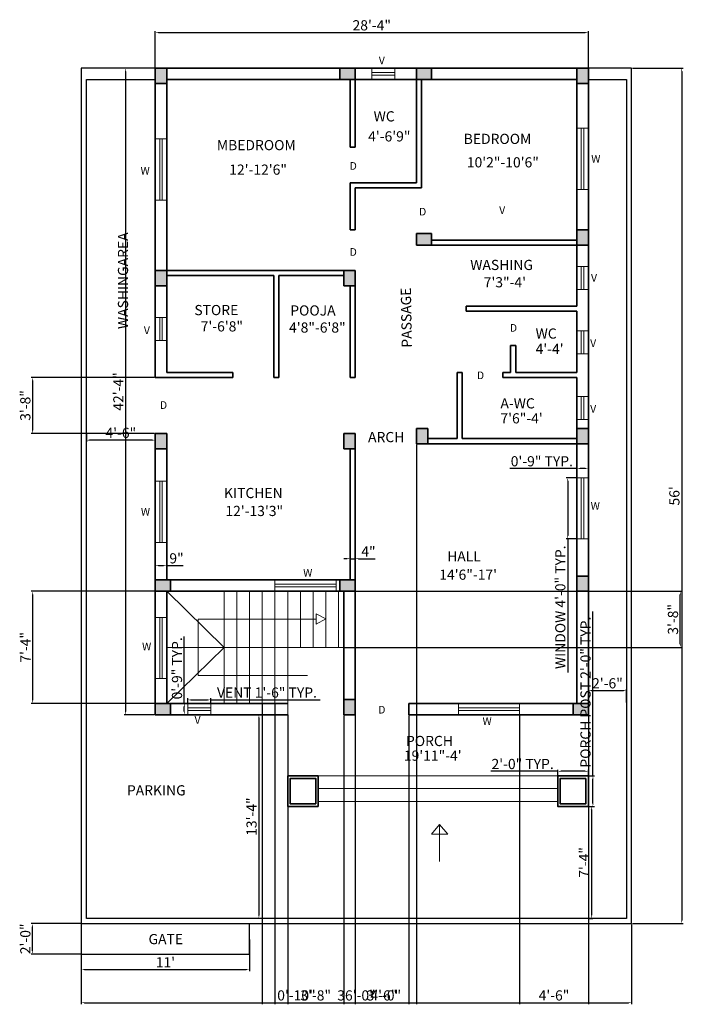
# Model space of a CAD drawing. Units: inches. Extents: x 2503 to 3024, y 1488 to 2262.
import ezdxf

# ---------------------------------------------------------------- set-up
doc = ezdxf.new("R2010")
doc.units = ezdxf.units.IN
for name, color, linetype, lineweight in [('A-ANNO-DIMS', 7, 'Continuous', 18), ('A-ANNO-SYMB', 121, 'Continuous', 18), ('A-ANNO-TEXT', 2, 'Continuous', 18), ('A-AREA-IDEN', 2, 'Continuous', 18), ('A-COLS', 121, 'Continuous', 35), ('A-COLS-PATT', 240, 'Continuous', 13), ('A-FLOR', 121, 'Continuous', 25), ('A-FLOR-STRS', 121, 'Continuous', 18), ('A-GLAZ', 6, 'Continuous', 18), ('A-WALL', 121, 'Continuous', 35), ('C-PROP', 121, 'Continuous', 25), ('C-SITE-GATE', 121, 'Continuous', 25)]:
    doc.layers.add(name, color=color, linetype=linetype, lineweight=lineweight)
doc.styles.get("Standard").update_dxf_attribs({"font": 'arial.ttf'})
doc.dimstyles.new('ISO-25', dxfattribs={"dimtxt": 8, "dimasz": 2.5, "dimexe": 1.25, "dimexo": 0.625, "dimtad": 1, "dimdec": 0, "dimlunit": 3, "dimtxsty": 'Standard', "dimcen": 2.5, "dimadec": 0, "dimazin": 0, "dimtfac": 1, "dimtdec": 0, "dimtmove": 0, "dimatfit": 3, "dimfxl": 1, "dimarcsym": 0})

# ---------------------------------------------------------------- blocks, each defined once
blk = doc.blocks.new('*D1')
at = {"layer": 'A-ANNO-DIMS', "color": 0, "lineweight": -2, "transparency": 16777216}
for p, q in [((2609.44, 2224.16), (2609.44, 2252.71)), ((2611.94, 2251.46), (2946.94, 2251.46)), ((2949.44, 2224.16), (2949.44, 2252.71))]:
    blk.add_line(p, q, dxfattribs=at)
at = {"layer": 'A-ANNO-DIMS', "color": 0, "transparency": 16777216}
for points in [[(2611.94, 2251.87), (2611.94, 2251.04), (2609.44, 2251.46)], [(2946.94, 2251.87), (2946.94, 2251.04), (2949.44, 2251.46)]]:
    blk.add_solid(points, dxfattribs=at)
at = {"layer": 'Defpoints', "color": 0, "transparency": 16777216}
for p in [(2949.44, 2251.46), (2609.44, 2223.53), (2949.44, 2223.53)]:
    blk.add_point(p, dxfattribs=at)
at = {"layer": 'A-ANNO-DIMS', "color": 0, "transparency": 16777216, "insert": (2779.44, 2256.17), "char_height": 8, "attachment_point": 5}
blk.add_mtext('28\'-4"', dxfattribs=at)
blk = doc.blocks.new('*D2')
at = {"layer": 'A-ANNO-DIMS', "color": 0, "lineweight": -2, "transparency": 16777216}
for p, q in [((2608.81, 2223.53), (2584.96, 2223.53)), ((2586.21, 2221.03), (2586.21, 1718.03)), ((2608.81, 1715.53), (2584.96, 1715.53))]:
    blk.add_line(p, q, dxfattribs=at)
at = {"layer": 'A-ANNO-DIMS', "color": 0, "transparency": 16777216}
for points in [[(2585.79, 2221.03), (2586.63, 2221.03), (2586.21, 2223.53)], [(2585.79, 1718.03), (2586.63, 1718.03), (2586.21, 1715.53)]]:
    blk.add_solid(points, dxfattribs=at)
at = {"layer": 'Defpoints', "color": 0, "transparency": 16777216}
for p in [(2609.44, 2223.53), (2586.21, 1715.53), (2609.44, 1715.53)]:
    blk.add_point(p, dxfattribs=at)
at = {"layer": 'A-ANNO-DIMS', "color": 0, "transparency": 16777216, "insert": (2581.57, 1969.53), "char_height": 8, "attachment_point": 5, "rotation": 90}
blk.add_mtext('42\'-4"', dxfattribs=at)
blk = doc.blocks.new('*D3')
at = {"layer": 'A-ANNO-DIMS', "color": 0, "lineweight": -2, "transparency": 16777216}
for p, q in [((2555.44, 1935.91), (2555.44, 1930.03)), ((2609.44, 1935.91), (2609.44, 1930.03)), ((2606.94, 1931.28), (2557.94, 1931.28))]:
    blk.add_line(p, q, dxfattribs=at)
at = {"layer": 'A-ANNO-DIMS', "color": 0, "transparency": 16777216}
for points in [[(2557.94, 1931.7), (2557.94, 1930.87), (2555.44, 1931.28)], [(2606.94, 1931.7), (2606.94, 1930.87), (2609.44, 1931.28)]]:
    blk.add_solid(points, dxfattribs=at)
at = {"layer": 'Defpoints', "color": 0, "transparency": 16777216}
for p in [(2555.44, 1936.53), (2609.44, 1936.53), (2555.44, 1931.28)]:
    blk.add_point(p, dxfattribs=at)
at = {"layer": 'A-ANNO-DIMS', "color": 0, "transparency": 16777216, "insert": (2582.44, 1935.99), "char_height": 8, "attachment_point": 5}
blk.add_mtext('4\'-6"', dxfattribs=at)
blk = doc.blocks.new('*D4')
at = {"layer": 'A-ANNO-DIMS', "color": 0, "lineweight": -2, "transparency": 16777216}
for p, q in [((2700.37, 1715.53), (2689.58, 1715.53)), ((2690.83, 1713.03), (2690.83, 1558.03)), ((2700.37, 1555.53), (2689.58, 1555.53))]:
    blk.add_line(p, q, dxfattribs=at)
at = {"layer": 'A-ANNO-DIMS', "color": 0, "transparency": 16777216}
for points in [[(2690.41, 1713.03), (2691.24, 1713.03), (2690.83, 1715.53)], [(2690.41, 1558.03), (2691.24, 1558.03), (2690.83, 1555.53)]]:
    blk.add_solid(points, dxfattribs=at)
at = {"layer": 'Defpoints', "color": 0, "transparency": 16777216}
for p in [(2700.99, 1715.53), (2690.83, 1555.53), (2700.99, 1555.53)]:
    blk.add_point(p, dxfattribs=at)
at = {"layer": 'A-ANNO-DIMS', "color": 0, "transparency": 16777216, "insert": (2686.11, 1635.53), "char_height": 8, "attachment_point": 5, "rotation": 90}
blk.add_mtext('13\'-4"', dxfattribs=at)
blk = doc.blocks.new('*D5')
at = {"layer": 'A-ANNO-DIMS', "color": 0, "lineweight": -2, "transparency": 16777216}
for p, q in [((2551.44, 1538.91), (2551.44, 1514.18)), ((2683.44, 1538.91), (2683.44, 1514.18)), ((2553.94, 1515.43), (2680.94, 1515.43))]:
    blk.add_line(p, q, dxfattribs=at)
at = {"layer": 'A-ANNO-DIMS', "color": 0, "transparency": 16777216}
for points in [[(2553.94, 1515.84), (2553.94, 1515.01), (2551.44, 1515.43)], [(2680.94, 1515.84), (2680.94, 1515.01), (2683.44, 1515.43)]]:
    blk.add_solid(points, dxfattribs=at)
at = {"layer": 'Defpoints', "color": 0, "transparency": 16777216}
for p in [(2551.44, 1539.53), (2683.44, 1539.53), (2683.44, 1515.43)]:
    blk.add_point(p, dxfattribs=at)
at = {"layer": 'A-ANNO-DIMS', "color": 0, "transparency": 16777216, "insert": (2617.44, 1520.07), "char_height": 8, "attachment_point": 5}
blk.add_mtext("11'", dxfattribs=at)
blk = doc.blocks.new('*D6')
at = {"layer": 'A-ANNO-DIMS', "color": 0, "lineweight": -2, "transparency": 16777216}
for p, q in [((2950.06, 1643.53), (2953.05, 1643.53)), ((2951.8, 1641.03), (2951.8, 1558.03)), ((2950.06, 1555.53), (2953.05, 1555.53))]:
    blk.add_line(p, q, dxfattribs=at)
at = {"layer": 'A-ANNO-DIMS', "color": 0, "transparency": 16777216}
for points in [[(2951.38, 1641.03), (2952.21, 1641.03), (2951.8, 1643.53)], [(2951.38, 1558.03), (2952.21, 1558.03), (2951.8, 1555.53)]]:
    blk.add_solid(points, dxfattribs=at)
at = {"layer": 'Defpoints', "color": 0, "transparency": 16777216}
for p in [(2949.44, 1643.53), (2949.44, 1555.53), (2951.8, 1555.53)]:
    blk.add_point(p, dxfattribs=at)
at = {"layer": 'A-ANNO-DIMS', "color": 0, "transparency": 16777216, "insert": (2947.17, 1599.53), "char_height": 8, "attachment_point": 5, "rotation": 90}
blk.add_mtext('7\'-4"', dxfattribs=at)
blk = doc.blocks.new('*D7')
at = {"layer": 'A-ANNO-DIMS', "color": 0, "lineweight": -2, "transparency": 16777216}
for p, q in [((2984.06, 2223.53), (3023.98, 2223.53)), ((3022.73, 2221.03), (3022.73, 1554.03)), ((2984.06, 1551.53), (3023.98, 1551.53))]:
    blk.add_line(p, q, dxfattribs=at)
at = {"layer": 'A-ANNO-DIMS', "color": 0, "transparency": 16777216}
for points in [[(3022.31, 2221.03), (3023.14, 2221.03), (3022.73, 2223.53)], [(3022.31, 1554.03), (3023.14, 1554.03), (3022.73, 1551.53)]]:
    blk.add_solid(points, dxfattribs=at)
at = {"layer": 'Defpoints', "color": 0, "transparency": 16777216}
for p in [(2983.44, 2223.53), (2983.44, 1551.53), (3022.73, 1551.53)]:
    blk.add_point(p, dxfattribs=at)
at = {"layer": 'A-ANNO-DIMS', "color": 0, "transparency": 16777216, "insert": (3018.02, 1887.53), "char_height": 8, "attachment_point": 5, "rotation": 90}
blk.add_mtext("56'", dxfattribs=at)
blk = doc.blocks.new('*D8')
at = {"layer": 'A-ANNO-DIMS', "color": 0, "lineweight": -2, "transparency": 16777216}
for p, q in [((2949.44, 1725.16), (2949.44, 1735.79)), ((2951.94, 1734.54), (2976.94, 1734.54)), ((2979.44, 1725.16), (2979.44, 1735.79))]:
    blk.add_line(p, q, dxfattribs=at)
at = {"layer": 'A-ANNO-DIMS', "color": 0, "transparency": 16777216}
for points in [[(2951.94, 1734.95), (2951.94, 1734.12), (2949.44, 1734.54)], [(2976.94, 1734.95), (2976.94, 1734.12), (2979.44, 1734.54)]]:
    blk.add_solid(points, dxfattribs=at)
at = {"layer": 'Defpoints', "color": 0, "transparency": 16777216}
for p in [(2979.44, 1734.54), (2949.44, 1724.53), (2979.44, 1724.53)]:
    blk.add_point(p, dxfattribs=at)
at = {"layer": 'A-ANNO-DIMS', "color": 0, "transparency": 16777216, "insert": (2964.44, 1739.25), "char_height": 8, "attachment_point": 5}
blk.add_mtext('2\'-6"', dxfattribs=at)
blk = doc.blocks.new('*D9')
at = {"layer": 'A-ANNO-DIMS', "color": 0, "lineweight": -2, "transparency": 16777216}
for p, q in [((2759.94, 1838.17), (2757.44, 1838.17)), ((2762.44, 1840.03), (2762.44, 1836.92)), ((2762.44, 1838.17), (2766.44, 1838.17)), ((2766.44, 1840.03), (2766.44, 1836.92)), ((2768.94, 1838.17), (2782.2, 1838.17))]:
    blk.add_line(p, q, dxfattribs=at)
at = {"layer": 'A-ANNO-DIMS', "color": 0, "transparency": 16777216}
for points in [[(2759.94, 1838.59), (2759.94, 1837.75), (2762.44, 1838.17)], [(2768.94, 1838.59), (2768.94, 1837.75), (2766.44, 1838.17)]]:
    blk.add_solid(points, dxfattribs=at)
at = {"layer": 'Defpoints', "color": 0, "transparency": 16777216}
for p in [(2762.44, 1840.65), (2766.44, 1840.65), (2766.44, 1838.17)]:
    blk.add_point(p, dxfattribs=at)
at = {"layer": 'A-ANNO-DIMS', "color": 0, "transparency": 16777216, "insert": (2776.82, 1842.79), "char_height": 8, "attachment_point": 5}
blk.add_mtext('4"', dxfattribs=at)
blk = doc.blocks.new('*D10')
at = {"layer": 'A-ANNO-DIMS', "color": 0, "lineweight": -2, "transparency": 16777216}
for p, q in [((2609.44, 1837.54), (2609.44, 1831.46)), ((2618.44, 1837.54), (2618.44, 1831.46)), ((2611.94, 1832.71), (2615.94, 1832.71)), ((2618.44, 1832.71), (2631.38, 1832.71))]:
    blk.add_line(p, q, dxfattribs=at)
at = {"layer": 'A-ANNO-DIMS', "color": 0, "transparency": 16777216}
for points in [[(2611.94, 1833.12), (2611.94, 1832.29), (2609.44, 1832.71)], [(2615.94, 1833.12), (2615.94, 1832.29), (2618.44, 1832.71)]]:
    blk.add_solid(points, dxfattribs=at)
at = {"layer": 'Defpoints', "color": 0, "transparency": 16777216}
for p in [(2609.44, 1838.17), (2618.44, 1838.17), (2618.44, 1832.71)]:
    blk.add_point(p, dxfattribs=at)
at = {"layer": 'A-ANNO-DIMS', "color": 0, "transparency": 16777216, "insert": (2626.16, 1837.42), "char_height": 8, "attachment_point": 5}
blk.add_mtext('9"', dxfattribs=at)
blk = doc.blocks.new('WIN-48IN')
for p, q in [((0, 48), (9, 48)), ((3.5, 48), (3.5, 0)), ((5.5, 48), (5.5, 0)), ((0, 0), (9, 0))]:
    blk.add_line(p, q)
blk = doc.blocks.new('VENT-18IN')
for p, q in [((0, 9), (0, 0)), ((18, 9), (18, 0)), ((0, 5.5), (18, 5.5)), ((0, 3.5), (18, 3.5))]:
    blk.add_line(p, q)
blk = doc.blocks.new('PORCH-POST-24IN')
for points in [[(24, 0), (24, 24), (0, 24), (0, 0)], [(22, 2), (22, 22), (2, 22), (2, 2)]]:
    blk.add_lwpolyline(points, close=True)
blk = doc.blocks.new('*D14')
at = {"layer": 'A-ANNO-DIMS', "color": 0, "lineweight": -2, "transparency": 16777216}
for p, q in [((2939.81, 1901.76), (2931.99, 1901.76)), ((2933.24, 1899.26), (2933.24, 1856.26)), ((2939.81, 1853.76), (2931.99, 1853.76)), ((2933.24, 1853.76), (2933.24, 1748.78))]:
    blk.add_line(p, q, dxfattribs=at)
at = {"layer": 'A-ANNO-DIMS', "color": 0, "transparency": 16777216}
for points in [[(2932.82, 1899.26), (2933.65, 1899.26), (2933.24, 1901.76)], [(2932.82, 1856.26), (2933.65, 1856.26), (2933.24, 1853.76)]]:
    blk.add_solid(points, dxfattribs=at)
at = {"layer": 'Defpoints', "color": 0, "transparency": 16777216}
for p in [(2940.44, 1901.76), (2933.24, 1853.76), (2940.44, 1853.76)]:
    blk.add_point(p, dxfattribs=at)
at = {"layer": 'A-ANNO-DIMS', "color": 0, "transparency": 16777216, "insert": (2928.47, 1800.02), "char_height": 8, "attachment_point": 5, "rotation": 90}
blk.add_mtext('WINDOW 4\'-0" TYP.', dxfattribs=at)
blk = doc.blocks.new('*D15')
at = {"layer": 'A-ANNO-DIMS', "color": 0, "lineweight": -2, "transparency": 16777216}
for p, q in [((2940.44, 1908.96), (2887.92, 1908.96)), ((2940.44, 1902.39), (2940.44, 1910.21)), ((2946.94, 1908.96), (2942.94, 1908.96)), ((2949.44, 1902.39), (2949.44, 1910.21))]:
    blk.add_line(p, q, dxfattribs=at)
at = {"layer": 'A-ANNO-DIMS', "color": 0, "transparency": 16777216}
for points in [[(2942.94, 1909.38), (2942.94, 1908.55), (2940.44, 1908.96)], [(2946.94, 1909.38), (2946.94, 1908.55), (2949.44, 1908.96)]]:
    blk.add_solid(points, dxfattribs=at)
at = {"layer": 'Defpoints', "color": 0, "transparency": 16777216}
for p in [(2940.44, 1908.96), (2940.44, 1901.76), (2949.44, 1901.76)]:
    blk.add_point(p, dxfattribs=at)
at = {"layer": 'A-ANNO-DIMS', "color": 0, "transparency": 16777216, "insert": (2912.93, 1913.67), "char_height": 8, "attachment_point": 5}
blk.add_mtext('0\'-9" TYP.', dxfattribs=at)
blk = doc.blocks.new('*D16')
at = {"layer": 'A-ANNO-DIMS', "color": 0, "lineweight": -2, "transparency": 16777216}
for p, q in [((2635, 1725.16), (2635, 1728.48)), ((2637.5, 1727.23), (2650.5, 1727.23)), ((2653, 1725.16), (2653, 1728.48)), ((2653, 1727.23), (2738.84, 1727.23))]:
    blk.add_line(p, q, dxfattribs=at)
at = {"layer": 'A-ANNO-DIMS', "color": 0, "transparency": 16777216}
for points in [[(2637.5, 1727.65), (2637.5, 1726.82), (2635, 1727.23)], [(2650.5, 1727.65), (2650.5, 1726.82), (2653, 1727.23)]]:
    blk.add_solid(points, dxfattribs=at)
at = {"layer": 'Defpoints', "color": 0, "transparency": 16777216}
for p in [(2653, 1727.23), (2635, 1724.53), (2653, 1724.53)]:
    blk.add_point(p, dxfattribs=at)
at = {"layer": 'A-ANNO-DIMS', "color": 0, "transparency": 16777216, "insert": (2697.17, 1731.94), "char_height": 8, "attachment_point": 5}
blk.add_mtext('VENT 1\'-6" TYP.', dxfattribs=at)
blk = doc.blocks.new('*D17')
at = {"layer": 'A-ANNO-DIMS', "color": 0, "lineweight": -2, "transparency": 16777216}
for p, q in [((2632.3, 1724.53), (2632.3, 1777.05)), ((2634.38, 1724.53), (2631.05, 1724.53)), ((2632.3, 1718.03), (2632.3, 1722.03)), ((2634.38, 1715.53), (2631.05, 1715.53))]:
    blk.add_line(p, q, dxfattribs=at)
at = {"layer": 'A-ANNO-DIMS', "color": 0, "transparency": 16777216}
for points in [[(2631.88, 1722.03), (2632.72, 1722.03), (2632.3, 1724.53)], [(2631.88, 1718.03), (2632.72, 1718.03), (2632.3, 1715.53)]]:
    blk.add_solid(points, dxfattribs=at)
at = {"layer": 'Defpoints', "color": 0, "transparency": 16777216}
for p in [(2632.3, 1724.53), (2635, 1724.53), (2635, 1715.53)]:
    blk.add_point(p, dxfattribs=at)
at = {"layer": 'A-ANNO-DIMS', "color": 0, "transparency": 16777216, "insert": (2627.59, 1752.04), "char_height": 8, "attachment_point": 5, "rotation": 90}
blk.add_mtext('0\'-9" TYP.', dxfattribs=at)
blk = doc.blocks.new('*D18')
at = {"layer": 'A-ANNO-DIMS', "color": 0, "lineweight": -2, "transparency": 16777216}
for p, q in [((2953.04, 1667.53), (2953.04, 1796.65)), ((2950.06, 1667.53), (2954.29, 1667.53)), ((2953.04, 1646.03), (2953.04, 1665.03)), ((2950.06, 1643.53), (2954.29, 1643.53))]:
    blk.add_line(p, q, dxfattribs=at)
at = {"layer": 'A-ANNO-DIMS', "color": 0, "transparency": 16777216}
for points in [[(2952.62, 1665.03), (2953.45, 1665.03), (2953.04, 1667.53)], [(2952.62, 1646.03), (2953.45, 1646.03), (2953.04, 1643.53)]]:
    blk.add_solid(points, dxfattribs=at)
at = {"layer": 'Defpoints', "color": 0, "transparency": 16777216}
for p in [(2949.44, 1667.53), (2953.04, 1667.53), (2949.44, 1643.53)]:
    blk.add_point(p, dxfattribs=at)
at = {"layer": 'A-ANNO-DIMS', "color": 0, "transparency": 16777216, "insert": (2948.27, 1733.34), "char_height": 8, "attachment_point": 5, "rotation": 90}
blk.add_mtext('PORCH POST 2\'-0" TYP.', dxfattribs=at)
blk = doc.blocks.new('*D19')
at = {"layer": 'A-ANNO-DIMS', "color": 0, "lineweight": -2, "transparency": 16777216}
for p, q in [((2925.44, 1671.13), (2872.78, 1671.13)), ((2925.44, 1668.16), (2925.44, 1672.38)), ((2946.94, 1671.13), (2927.94, 1671.13)), ((2949.44, 1668.16), (2949.44, 1672.38))]:
    blk.add_line(p, q, dxfattribs=at)
at = {"layer": 'A-ANNO-DIMS', "color": 0, "transparency": 16777216}
for points in [[(2927.94, 1671.55), (2927.94, 1670.72), (2925.44, 1671.13)], [(2946.94, 1671.55), (2946.94, 1670.72), (2949.44, 1671.13)]]:
    blk.add_solid(points, dxfattribs=at)
at = {"layer": 'Defpoints', "color": 0, "transparency": 16777216}
for p in [(2925.44, 1671.13), (2925.44, 1667.53), (2949.44, 1667.53)]:
    blk.add_point(p, dxfattribs=at)
at = {"layer": 'A-ANNO-DIMS', "color": 0, "transparency": 16777216, "insert": (2897.86, 1675.84), "char_height": 8, "attachment_point": 5}
blk.add_mtext('2\'-0" TYP.', dxfattribs=at)
blk = doc.blocks.new('*D20')
at = {"layer": 'A-ANNO-DIMS', "color": 0, "lineweight": -2, "transparency": 16777216}
for p, q in [((2551.44, 1550.91), (2551.44, 1488.08)), ((2983.44, 1550.91), (2983.44, 1488.08)), ((2553.94, 1489.33), (2980.94, 1489.33))]:
    blk.add_line(p, q, dxfattribs=at)
at = {"layer": 'A-ANNO-DIMS', "color": 0, "transparency": 16777216}
for points in [[(2553.94, 1489.75), (2553.94, 1488.92), (2551.44, 1489.33)], [(2980.94, 1489.75), (2980.94, 1488.92), (2983.44, 1489.33)]]:
    blk.add_solid(points, dxfattribs=at)
at = {"layer": 'Defpoints', "color": 0, "transparency": 16777216}
for p in [(2551.44, 1551.53), (2983.44, 1551.53), (2983.44, 1489.33)]:
    blk.add_point(p, dxfattribs=at)
at = {"layer": 'A-ANNO-DIMS', "color": 0, "transparency": 16777216, "insert": (2767.44, 1494.05), "char_height": 8, "attachment_point": 5}
blk.add_mtext('36\'-0"', dxfattribs=at)
blk = doc.blocks.new('*D21')
at = {"layer": 'A-ANNO-DIMS', "color": 0, "lineweight": -2, "transparency": 16777216}
for p, q in [((2550.81, 1551.53), (2511.99, 1551.53)), ((2513.24, 1530.03), (2513.24, 1549.03)), ((2550.81, 1527.53), (2511.99, 1527.53))]:
    blk.add_line(p, q, dxfattribs=at)
at = {"layer": 'A-ANNO-DIMS', "color": 0, "transparency": 16777216}
for points in [[(2512.82, 1549.03), (2513.65, 1549.03), (2513.24, 1551.53)], [(2512.82, 1530.03), (2513.65, 1530.03), (2513.24, 1527.53)]]:
    blk.add_solid(points, dxfattribs=at)
at = {"layer": 'Defpoints', "color": 0, "transparency": 16777216}
for p in [(2513.24, 1551.53), (2551.44, 1551.53), (2551.44, 1527.53)]:
    blk.add_point(p, dxfattribs=at)
at = {"layer": 'A-ANNO-DIMS', "color": 0, "transparency": 16777216, "insert": (2508.53, 1539.53), "char_height": 8, "attachment_point": 5, "rotation": 90}
blk.add_mtext('2\'-0"', dxfattribs=at)
blk = doc.blocks.new('*D22')
at = {"layer": 'A-ANNO-DIMS', "color": 0, "lineweight": -2, "transparency": 16777216}
for p, q in [((2617.81, 1812.53), (2511.99, 1812.53)), ((2513.24, 1810.03), (2513.24, 1727.03)), ((2617.81, 1724.53), (2511.99, 1724.53))]:
    blk.add_line(p, q, dxfattribs=at)
at = {"layer": 'A-ANNO-DIMS', "color": 0, "transparency": 16777216}
for points in [[(2512.82, 1810.03), (2513.65, 1810.03), (2513.24, 1812.53)], [(2512.82, 1727.03), (2513.65, 1727.03), (2513.24, 1724.53)]]:
    blk.add_solid(points, dxfattribs=at)
at = {"layer": 'Defpoints', "color": 0, "transparency": 16777216}
for p in [(2618.44, 1812.53), (2513.24, 1724.53), (2618.44, 1724.53)]:
    blk.add_point(p, dxfattribs=at)
at = {"layer": 'A-ANNO-DIMS', "color": 0, "transparency": 16777216, "insert": (2508.61, 1768.53), "char_height": 8, "attachment_point": 5, "rotation": 90}
blk.add_mtext('7\'-4"', dxfattribs=at)
blk = doc.blocks.new('*D23')
at = {"layer": 'A-ANNO-DIMS', "color": 0, "lineweight": -2, "transparency": 16777216}
for p, q in [((2758.06, 1812.53), (3022.89, 1812.53)), ((3021.64, 1771.03), (3021.64, 1810.03)), ((2758.06, 1768.53), (3022.89, 1768.53))]:
    blk.add_line(p, q, dxfattribs=at)
at = {"layer": 'A-ANNO-DIMS', "color": 0, "transparency": 16777216}
for points in [[(3021.22, 1810.03), (3022.05, 1810.03), (3021.64, 1812.53)], [(3021.22, 1771.03), (3022.05, 1771.03), (3021.64, 1768.53)]]:
    blk.add_solid(points, dxfattribs=at)
at = {"layer": 'Defpoints', "color": 0, "transparency": 16777216}
for p in [(2757.44, 1812.53), (3021.64, 1812.53), (2757.44, 1768.53)]:
    blk.add_point(p, dxfattribs=at)
at = {"layer": 'A-ANNO-DIMS', "color": 0, "transparency": 16777216, "insert": (3016.92, 1790.53), "char_height": 8, "attachment_point": 5, "rotation": 90}
blk.add_mtext('3\'-8"', dxfattribs=at)
blk = doc.blocks.new('*D24')
at = {"layer": 'A-ANNO-DIMS', "color": 0, "lineweight": -2, "transparency": 16777216}
for p, q in [((2608.81, 1980.53), (2511.99, 1980.53)), ((2513.24, 1978.03), (2513.24, 1939.03)), ((2608.81, 1936.53), (2511.99, 1936.53))]:
    blk.add_line(p, q, dxfattribs=at)
at = {"layer": 'A-ANNO-DIMS', "color": 0, "transparency": 16777216}
for points in [[(2512.82, 1978.03), (2513.65, 1978.03), (2513.24, 1980.53)], [(2512.82, 1939.03), (2513.65, 1939.03), (2513.24, 1936.53)]]:
    blk.add_solid(points, dxfattribs=at)
at = {"layer": 'Defpoints', "color": 0, "transparency": 16777216}
for p in [(2609.44, 1980.53), (2513.24, 1936.53), (2609.44, 1936.53)]:
    blk.add_point(p, dxfattribs=at)
at = {"layer": 'A-ANNO-DIMS', "color": 0, "transparency": 16777216, "insert": (2508.52, 1958.53), "char_height": 8, "attachment_point": 5, "rotation": 90}
blk.add_mtext('3\'-8"', dxfattribs=at)
blk = doc.blocks.new('*D25')
at = {"layer": 'A-ANNO-DIMS', "color": 0, "lineweight": -2, "transparency": 16777216}
for p, q in [((2766.44, 1714.91), (2766.44, 1488.08)), ((2808.44, 1714.91), (2808.44, 1488.08)), ((2768.94, 1489.33), (2805.94, 1489.33))]:
    blk.add_line(p, q, dxfattribs=at)
at = {"layer": 'A-ANNO-DIMS', "color": 0, "transparency": 16777216}
for points in [[(2768.94, 1489.75), (2768.94, 1488.92), (2766.44, 1489.33)], [(2805.94, 1489.75), (2805.94, 1488.92), (2808.44, 1489.33)]]:
    blk.add_solid(points, dxfattribs=at)
at = {"layer": 'Defpoints', "color": 0, "transparency": 16777216}
for p in [(2766.44, 1715.53), (2808.44, 1715.53), (2808.44, 1489.33)]:
    blk.add_point(p, dxfattribs=at)
at = {"layer": 'A-ANNO-DIMS', "color": 0, "transparency": 16777216, "insert": (2787.44, 1494.05), "char_height": 8, "attachment_point": 5}
blk.add_mtext('3\'-6"', dxfattribs=at)
blk = doc.blocks.new('*D26')
at = {"layer": 'A-ANNO-DIMS', "color": 0, "lineweight": -2, "transparency": 16777216}
for p, q in [((2814.44, 1927.91), (2814.44, 1488.08)), ((2766.44, 1923.91), (2766.44, 1488.08)), ((2768.94, 1489.33), (2811.94, 1489.33))]:
    blk.add_line(p, q, dxfattribs=at)
at = {"layer": 'A-ANNO-DIMS', "color": 0, "transparency": 16777216}
for points in [[(2768.94, 1489.75), (2768.94, 1488.92), (2766.44, 1489.33)], [(2811.94, 1489.75), (2811.94, 1488.92), (2814.44, 1489.33)]]:
    blk.add_solid(points, dxfattribs=at)
at = {"layer": 'Defpoints', "color": 0, "transparency": 16777216}
for p in [(2814.44, 1928.53), (2766.44, 1924.53), (2814.44, 1489.33)]:
    blk.add_point(p, dxfattribs=at)
at = {"layer": 'A-ANNO-DIMS', "color": 0, "transparency": 16777216, "insert": (2790.44, 1494.04), "char_height": 8, "attachment_point": 5}
blk.add_mtext('4\'-0"', dxfattribs=at)
blk = doc.blocks.new('*D27')
at = {"layer": 'A-ANNO-DIMS', "color": 0, "lineweight": -2, "transparency": 16777216}
for p, q in [((2713.44, 1714.91), (2713.44, 1488.08)), ((2757.44, 1714.91), (2757.44, 1488.08)), ((2715.94, 1489.33), (2754.94, 1489.33))]:
    blk.add_line(p, q, dxfattribs=at)
at = {"layer": 'A-ANNO-DIMS', "color": 0, "transparency": 16777216}
for points in [[(2715.94, 1489.75), (2715.94, 1488.92), (2713.44, 1489.33)], [(2754.94, 1489.75), (2754.94, 1488.92), (2757.44, 1489.33)]]:
    blk.add_solid(points, dxfattribs=at)
at = {"layer": 'Defpoints', "color": 0, "transparency": 16777216}
for p in [(2713.44, 1715.53), (2757.44, 1715.53), (2757.44, 1489.33)]:
    blk.add_point(p, dxfattribs=at)
at = {"layer": 'A-ANNO-DIMS', "color": 0, "transparency": 16777216, "insert": (2735.44, 1494.05), "char_height": 8, "attachment_point": 5}
blk.add_mtext('3\'-8"', dxfattribs=at)
blk = doc.blocks.new('*D28')
at = {"layer": 'A-ANNO-DIMS', "color": 0, "lineweight": -2, "transparency": 16777216}
for p, q in [((2693.44, 1723.91), (2693.44, 1488.08)), ((2703.44, 1723.91), (2703.44, 1488.08)), ((2695.94, 1489.33), (2700.94, 1489.33)), ((2703.44, 1489.33), (2734.67, 1489.33))]:
    blk.add_line(p, q, dxfattribs=at)
at = {"layer": 'A-ANNO-DIMS', "color": 0, "transparency": 16777216}
for points in [[(2695.94, 1489.75), (2695.94, 1488.92), (2693.44, 1489.33)], [(2700.94, 1489.75), (2700.94, 1488.92), (2703.44, 1489.33)]]:
    blk.add_solid(points, dxfattribs=at)
at = {"layer": 'Defpoints', "color": 0, "transparency": 16777216}
for p in [(2693.44, 1724.53), (2703.44, 1724.53), (2703.44, 1489.33)]:
    blk.add_point(p, dxfattribs=at)
at = {"layer": 'A-ANNO-DIMS', "color": 0, "transparency": 16777216, "insert": (2720.3, 1494.04), "char_height": 8, "attachment_point": 5}
blk.add_mtext('0\'-10"', dxfattribs=at)
blk = doc.blocks.new('*D29')
at = {"layer": 'A-ANNO-DIMS', "color": 0, "lineweight": -2, "transparency": 16777216}
for p, q in [((2895.5, 1714.91), (2895.5, 1488.08)), ((2949.44, 1714.91), (2949.44, 1488.08)), ((2898, 1489.33), (2946.94, 1489.33))]:
    blk.add_line(p, q, dxfattribs=at)
at = {"layer": 'A-ANNO-DIMS', "color": 0, "transparency": 16777216}
for points in [[(2898, 1489.75), (2898, 1488.92), (2895.5, 1489.33)], [(2946.94, 1489.75), (2946.94, 1488.92), (2949.44, 1489.33)]]:
    blk.add_solid(points, dxfattribs=at)
at = {"layer": 'Defpoints', "color": 0, "transparency": 16777216}
for p in [(2895.5, 1715.53), (2949.44, 1715.53), (2949.44, 1489.33)]:
    blk.add_point(p, dxfattribs=at)
at = {"layer": 'A-ANNO-DIMS', "color": 0, "transparency": 16777216, "insert": (2922.47, 1494.04), "char_height": 8, "attachment_point": 5}
blk.add_mtext('4\'-6"', dxfattribs=at)

msp = doc.modelspace()

# ---------------------------------------------------------------- hatches: boundary and pattern name
at = {"layer": 'A-COLS-PATT'}
h = msp.add_hatch(color=256, dxfattribs=at)
h.dxf.hatch_style = 1
h.paths.add_polyline_path([(2618.44, 2223.53), (2609.44, 2223.53), (2609.44, 2211.53), (2618.44, 2211.53)])
h = msp.add_hatch(color=256, dxfattribs=at)
h.dxf.hatch_style = 1
h.paths.add_polyline_path([(2766.44, 2223.53), (2754.44, 2223.53), (2754.44, 2214.53), (2766.44, 2214.53)])
h = msp.add_hatch(color=256, dxfattribs=at)
h.dxf.hatch_style = 1
h.paths.add_polyline_path([(2826.44, 2223.53), (2814.44, 2223.53), (2814.44, 2214.53), (2826.44, 2214.53)])
h = msp.add_hatch(color=256, dxfattribs=at)
h.dxf.hatch_style = 1
h.paths.add_polyline_path([(2949.44, 2223.53), (2940.44, 2223.53), (2940.44, 2211.53), (2949.44, 2211.53)])
h = msp.add_hatch(color=256, dxfattribs=at)
h.dxf.hatch_style = 1
h.paths.add_polyline_path([(2949.44, 2096.53), (2940.44, 2096.53), (2940.44, 2084.53), (2949.44, 2084.53)])
h = msp.add_hatch(color=256, dxfattribs=at)
h.dxf.hatch_style = 1
h.paths.add_polyline_path([(2826.44, 2093.53), (2814.44, 2093.53), (2814.44, 2088.53), (2814.44, 2084.53), (2826.44, 2084.53)])
h = msp.add_hatch(color=256, dxfattribs=at)
h.dxf.hatch_style = 1
h.paths.add_polyline_path([(2618.44, 2064.53), (2609.44, 2064.53), (2609.44, 2052.53), (2618.44, 2052.53)])
h = msp.add_hatch(color=256, dxfattribs=at)
h.dxf.hatch_style = 1
h.paths.add_polyline_path([(2766.44, 2064.53), (2757.44, 2064.53), (2757.44, 2052.53), (2766.44, 2052.53)])
h = msp.add_hatch(color=256, dxfattribs=at)
h.dxf.hatch_style = 1
h.paths.add_polyline_path([(2618.44, 1936.53), (2609.44, 1936.53), (2609.44, 1924.53), (2618.44, 1924.53)])
h = msp.add_hatch(color=256, dxfattribs=at)
h.dxf.hatch_style = 1
h.paths.add_polyline_path([(2766.44, 1936.53), (2762.44, 1936.53), (2757.44, 1936.53), (2757.44, 1924.53), (2766.44, 1924.53)])
h = msp.add_hatch(color=256, dxfattribs=at)
h.dxf.hatch_style = 1
h.paths.add_polyline_path([(2823.44, 1940.53), (2814.44, 1940.53), (2814.44, 1932.53), (2814.44, 1928.53), (2823.44, 1928.53)])
h = msp.add_hatch(color=256, dxfattribs=at)
h.dxf.hatch_style = 1
h.paths.add_polyline_path([(2949.44, 1940.53), (2940.44, 1940.53), (2940.44, 1928.53), (2949.44, 1928.53)])
h = msp.add_hatch(color=256, dxfattribs=at)
h.dxf.hatch_style = 1
h.paths.add_polyline_path([(2621.44, 1821.53), (2609.44, 1821.53), (2609.44, 1812.53), (2621.44, 1812.53)])
h = msp.add_hatch(color=256, dxfattribs=at)
h.dxf.hatch_style = 1
h.paths.add_polyline_path([(2766.44, 1821.53), (2754.44, 1821.53), (2754.44, 1812.53), (2757.44, 1812.53), (2766.44, 1812.53)])
h = msp.add_hatch(color=256, dxfattribs=at)
h.dxf.hatch_style = 1
h.paths.add_polyline_path([(2949.44, 1824.53), (2940.44, 1824.53), (2940.44, 1812.53), (2949.44, 1812.53)])
h = msp.add_hatch(color=256, dxfattribs=at)
h.dxf.hatch_style = 1
h.paths.add_polyline_path([(2766.44, 1727.53), (2757.44, 1727.53), (2757.44, 1715.53), (2766.44, 1715.53)])
h = msp.add_hatch(color=256, dxfattribs=at)
h.dxf.hatch_style = 1
h.paths.add_polyline_path([(2621.44, 1724.53), (2609.44, 1724.53), (2609.44, 1715.53), (2621.44, 1715.53)])
h = msp.add_hatch(color=256, dxfattribs=at)
h.dxf.hatch_style = 1
h.paths.add_polyline_path([(2949.44, 1724.53), (2937.44, 1724.53), (2937.44, 1715.53), (2949.44, 1715.53)])

# ---------------------------------------------------------------- linework, layer by layer
at = {"layer": 'A-ANNO-SYMB'}
for p, q in [((2735.74, 1790.77), (2735.74, 1794.77)), ((2743.44, 1790.87), (2735.74, 1794.77)), ((2643.15, 1746.53), (2643.15, 1790.77)), ((2643.15, 1790.77), (2735.74, 1790.77)), ((2735.74, 1786.77), (2743.44, 1790.87)), ((2735.74, 1790.77), (2735.74, 1786.77)), ((2729.02, 1746.53), (2643.15, 1746.53)), ((2832.68, 1629.35), (2826.25, 1621.69)), ((2832.68, 1629.35), (2832.68, 1600.22)), ((2832.68, 1629.35), (2839.1, 1621.69)), ((2839.1, 1621.69), (2826.25, 1621.69))]:
    msp.add_line(p, q, dxfattribs=at)
at = {"layer": 'A-COLS'}
for p, q in [((2754.44, 2223.53), (2754.44, 2214.53)), ((2826.44, 2223.53), (2826.44, 2214.53)), ((2609.44, 2211.53), (2618.44, 2211.53)), ((2940.44, 2211.53), (2949.44, 2211.53)), ((2949.44, 2096.53), (2940.44, 2096.53)), ((2814.44, 2088.53), (2814.44, 2093.53)), ((2814.44, 2093.53), (2826.44, 2093.53)), ((2826.44, 2093.53), (2826.44, 2084.53)), ((2814.44, 2084.53), (2814.44, 2088.53)), ((2766.44, 2064.53), (2757.44, 2064.53)), ((2757.44, 2064.53), (2757.44, 2052.53)), ((2609.44, 2052.53), (2618.44, 2052.53)), ((2757.44, 2052.53), (2766.44, 2052.53)), ((2609.44, 1936.53), (2618.44, 1936.53)), ((2762.44, 1936.53), (2757.44, 1936.53)), ((2757.44, 1936.53), (2757.44, 1924.53)), ((2762.44, 1936.53), (2766.44, 1936.53)), ((2814.44, 1932.53), (2814.44, 1940.53)), ((2814.44, 1940.53), (2823.44, 1940.53)), ((2823.44, 1940.53), (2823.44, 1928.53)), ((2949.44, 1940.53), (2940.44, 1940.53)), ((2814.44, 1932.53), (2814.44, 1928.53)), ((2609.44, 1924.53), (2618.44, 1924.53)), ((2757.44, 1924.53), (2766.44, 1924.53)), ((2621.44, 1821.53), (2621.44, 1812.53)), ((2754.44, 1821.53), (2754.44, 1812.53)), ((2940.44, 1824.53), (2949.44, 1824.53)), ((2757.44, 1812.53), (2753.44, 1812.53)), ((2940.44, 1812.53), (2949.44, 1812.53)), ((2757.44, 1727.53), (2766.44, 1727.53)), ((2621.44, 1724.53), (2621.44, 1715.53)), ((2937.44, 1715.53), (2937.44, 1724.53))]:
    msp.add_line(p, q, dxfattribs=at)
msp.add_lwpolyline([(2766.44, 1715.53), (2757.44, 1715.53)], dxfattribs=at)
at = {"layer": 'A-FLOR'}
for p, q in [((2713.44, 1715.53), (2713.44, 1667.53)), ((2949.44, 1715.53), (2949.44, 1667.53))]:
    msp.add_line(p, q, dxfattribs=at)
at = {"layer": 'A-FLOR-STRS'}
for p, q in [((2618.44, 1812.53), (2663.44, 1768.53)), ((2663.44, 1812.53), (2663.44, 1724.53)), ((2673.44, 1812.53), (2673.44, 1724.53)), ((2683.44, 1812.53), (2683.44, 1724.53)), ((2693.44, 1812.53), (2693.44, 1724.53)), ((2703.44, 1812.53), (2703.44, 1724.53)), ((2713.44, 1812.53), (2713.44, 1715.53)), ((2723.44, 1812.53), (2723.44, 1768.53)), ((2733.44, 1812.53), (2733.44, 1768.53)), ((2743.44, 1812.53), (2743.44, 1768.53)), ((2753.44, 1812.53), (2753.44, 1768.53)), ((2618.44, 1768.53), (2757.44, 1768.53)), ((2663.44, 1768.53), (2618.44, 1724.53)), ((2737.44, 1667.53), (2925.44, 1667.53)), ((2737.44, 1657.53), (2925.44, 1657.53)), ((2737.44, 1647.53), (2925.44, 1647.53))]:
    msp.add_line(p, q, dxfattribs=at)
at = {"layer": 'A-WALL'}
for p, q in [((2618.44, 1984.53), (2618.44, 2223.53)), ((2766.44, 2161.53), (2766.44, 2223.53)), ((2814.44, 2133.53), (2814.44, 2223.53)), ((2940.44, 2223.53), (2940.44, 2036.53)), ((2618.44, 2214.53), (2940.44, 2214.53)), ((2762.44, 2161.53), (2762.44, 2214.53)), ((2818.44, 2129.53), (2818.44, 2214.53)), ((2762.44, 2161.53), (2766.44, 2161.53)), ((2762.44, 2133.53), (2814.44, 2133.53)), ((2762.44, 2096.53), (2762.44, 2133.53)), ((2766.44, 2129.53), (2818.44, 2129.53)), ((2766.44, 2096.53), (2766.44, 2129.53)), ((2762.44, 2096.53), (2766.44, 2096.53)), ((2814.44, 2084.53), (2949.44, 2084.53)), ((2826.44, 2088.53), (2940.44, 2088.53)), ((2609.44, 2064.53), (2766.44, 2064.53)), ((2618.44, 2060.53), (2702.44, 2060.53)), ((2702.44, 1980.53), (2702.44, 2060.53)), ((2706.44, 1980.53), (2706.44, 2060.53)), ((2706.44, 2060.53), (2757.44, 2060.53)), ((2766.44, 1980.53), (2766.44, 2064.53)), ((2762.44, 1980.53), (2762.44, 2052.53)), ((2853.44, 2036.53), (2940.44, 2036.53)), ((2853.44, 2036.53), (2853.44, 2032.53)), ((2853.44, 2032.53), (2940.44, 2032.53)), ((2940.44, 2032.53), (2940.44, 1984.53)), ((2888.44, 2005.53), (2888.44, 1984.53)), ((2888.44, 2005.53), (2892.44, 2005.53)), ((2892.44, 2005.53), (2892.44, 1984.53)), ((2618.44, 1980.53), (2609.44, 1980.53)), ((2618.44, 1984.53), (2670.44, 1984.53)), ((2618.44, 1980.53), (2670.44, 1980.53)), ((2670.44, 1980.53), (2670.44, 1984.53)), ((2702.44, 1980.53), (2706.44, 1980.53)), ((2762.44, 1980.53), (2766.44, 1980.53)), ((2846.44, 1984.53), (2850.44, 1984.53)), ((2846.44, 1984.53), (2846.44, 1932.53)), ((2850.44, 1984.53), (2850.44, 1932.53)), ((2882.44, 1984.53), (2882.44, 1980.53)), ((2882.44, 1984.53), (2888.44, 1984.53)), ((2882.44, 1980.53), (2940.44, 1980.53)), ((2892.44, 1984.53), (2940.44, 1984.53)), ((2940.44, 1980.53), (2940.44, 1724.53)), ((2618.44, 1821.53), (2618.44, 1936.53)), ((2766.44, 1715.53), (2766.44, 1936.53)), ((2814.44, 1928.53), (2949.44, 1928.53)), ((2823.44, 1932.53), (2846.44, 1932.53)), ((2850.44, 1932.53), (2940.44, 1932.53)), ((2762.44, 1821.53), (2762.44, 1924.53)), ((2609.44, 1821.53), (2766.44, 1821.53)), ((2609.44, 1812.53), (2766.44, 1812.53)), ((2618.44, 1724.53), (2618.44, 1812.53)), ((2757.44, 1715.53), (2757.44, 1812.53)), ((2713.44, 1724.53), (2609.44, 1724.53)), ((2949.44, 1724.53), (2808.44, 1724.53)), ((2808.44, 1715.53), (2808.44, 1724.53))]:
    msp.add_line(p, q, dxfattribs=at)
for points in [[(2609.44, 1980.53), (2609.44, 2223.53), (2949.44, 2223.53), (2949.44, 1715.53), (2808.44, 1715.53)], [(2713.44, 1715.53), (2609.44, 1715.53), (2609.44, 1936.53)]]:
    msp.add_lwpolyline(points, dxfattribs=at)
at = {"layer": 'C-PROP'}
for p, q in [((2609.44, 2223.53), (2551.44, 2223.53)), ((2551.44, 2223.53), (2551.44, 1551.53)), ((2983.44, 2223.53), (2949.44, 2223.53)), ((2983.44, 1551.53), (2983.44, 2223.53)), ((2555.44, 1555.53), (2555.44, 2214.53)), ((2555.44, 2214.53), (2609.44, 2214.53)), ((2949.44, 2214.53), (2979.44, 2214.53)), ((2979.44, 2214.53), (2979.44, 1555.53)), ((2979.44, 1555.53), (2555.44, 1555.53)), ((2551.44, 1551.53), (2609.44, 1551.53)), ((2609.44, 1551.53), (2949.44, 1551.53)), ((2949.44, 1551.53), (2983.44, 1551.53))]:
    msp.add_line(p, q, dxfattribs=at)
at = {"layer": 'C-SITE-GATE'}
for p, q in [((2551.44, 1551.53), (2551.44, 1527.53)), ((2683.44, 1527.53), (2683.44, 1551.53)), ((2551.44, 1527.53), (2683.44, 1527.53))]:
    msp.add_line(p, q, dxfattribs=at)

# ---------------------------------------------------------------- block references
at = {"layer": 'A-COLS'}
msp.add_blockref('PORCH-POST-24IN', (2713.44, 1643.53), dxfattribs=at)
at = {"layer": 'A-COLS', "rotation": 90.0000000000009}
msp.add_blockref('PORCH-POST-24IN', (2949.44, 1643.53), dxfattribs=at)
at = {"layer": 'A-GLAZ'}
for name, p in [('VENT-18IN', (2779.44, 2214.53)), ('WIN-48IN', (2609.44, 2119.9)), ('VENT-18IN', (2635, 1715.53))]:
    msp.add_blockref(name, p, dxfattribs=at)
for name, p, rotation in [('WIN-48IN', (2949.44, 2176.28), 180), ('VENT-18IN', (2949.44, 2049.74), 90.00000000000236), ('VENT-18IN', (2618.44, 2009.57), 90.00000000000236), ('VENT-18IN', (2949.44, 1999.11), 90.00000000000236), ('VENT-18IN', (2940.44, 1965.56), 270.0000000000017), ('WIN-48IN', (2618.44, 1898.97), 180), ('WIN-48IN', (2949.44, 1901.76), 180), ('WIN-48IN', (2751.44, 1812.53), 89.99999999999895), ('WIN-48IN', (2618.44, 1792), 180), ('WIN-48IN', (2895.5, 1715.53), 89.99999999999913)]:
    msp.add_blockref(name, p, dxfattribs=dict(at, rotation=rotation))

# ---------------------------------------------------------------- texts
at = {"layer": 'A-ANNO-TEXT'}
for tag, p, height in [('V', (2784.96, 2226.58), 6), ('W', (2951.72, 2149.27), 6), ('W', (2597.94, 2139.98), 6), ('D', (2762.08, 2143.73), 6), ('D', (2816.56, 2107.79), 6), ('V', (2879.46, 2109.03), 6), ('D', (2762.08, 2076.13), 6), ('V', (2951.54, 2055.79), 6), ('V', (2600.54, 2014.59), 6), ('D', (2887.84, 2016.49), 6), ('V', (2950.87, 2004.57), 6), ('D', (2862, 1979.22), 6), ('D', (2613.17, 1955.85), 6), ('V', (2950.89, 1952.88), 6), ('ARCH', (2776.52, 1929.71), 8), ('W', (2951.29, 1876.59), 6), ('W', (2598.21, 1872.04), 6), ('W', (2725.61, 1824.08), 6), ('W', (2599.14, 1766.15), 6), ('D', (2784.52, 1716.54), 6), ('V', (2640.31, 1708.48), 6), ('W', (2866.38, 1707.58), 6), ('GATE', (2604.19, 1535.31), 8)]:
    msp.add_attdef(tag, p, '', height=height, dxfattribs=at)
at = {"layer": 'A-AREA-IDEN'}
for tag, p in [('WC', (2780.88, 2181.68)), ('4\'-6\'9"', (2776.6, 2165.95)), ('MBEDROOM', (2657.81, 2159.07)), ('BEDROOM', (2851.62, 2163.99)), ('10\'2"-10\'6"', (2854.06, 2145.56)), ('12\'-12\'6"', (2667.55, 2139.82)), ('WASHING', (2856.74, 2064.95)), ('7\'3"-4\'', (2867.33, 2051.34)), ('STORE', (2640.16, 2029.49)), ('POOJA', (2715.46, 2029.17)), ('7\'-6\'8"', (2645.16, 2016.69)), ('4\'8"-6\'8"', (2714.52, 2015.75)), ('WC', (2908.05, 2011.05)), ("4'-4'", (2908.05, 1999)), ('A-WC', (2880.44, 1956.2)), ('7\'6"-4\'', (2880.44, 1944.46)), ('KITCHEN', (2663.48, 1885.76)), ('12\'-13\'3"', (2664.53, 1871.67)), ('HALL', (2838.62, 1836.02)), ('14\'6"-17\'', (2832.43, 1821.61)), ('PORCH', (2806.3, 1690.97)), ('19\'11"-4\'', (2804.64, 1679.41)), ('PARKING', (2587.24, 1652.2))]:
    msp.add_attdef(tag, p, '', height=8, dxfattribs=at)
for tag, p, rotation in [('WASHINGAREA', (2588.16, 2018.57), 90), ('PASSAGE', (2810.98, 2004.04), 91.01785)]:
    msp.add_attdef(tag, p, '', height=8, rotation=rotation, dxfattribs=at)

# ---------------------------------------------------------------- dimensions: what is measured, and where the dimension line sits
at = {"layer": 'A-ANNO-DIMS'}
for base, p1, p2, override, picture, middle in [((2949.44, 2251.46), (2609.44, 2223.53), (2949.44, 2223.53), {"dimclrd": 0, "dimclre": 0, "dimclrt": 0}, '*D1', (2779.44, 2256.17)), ((2555.44, 1931.28), (2609.44, 1936.53), (2555.44, 1936.53), {"dimclrd": 0, "dimclre": 0, "dimclrt": 0}, '*D3', (2582.44, 1935.99)), ((2814.44, 1489.33), (2766.44, 1924.53), (2814.44, 1928.53), {"dimdec": 1, "dimlfac": 1, "dimrnd": 0, "dimzin": 1, "dimdsep": 46, "dimlunit": 4, "dimfrac": 2}, '*D26', (2790.44, 1494.04)), ((2618.44, 1832.71), (2609.44, 1838.17), (2618.44, 1838.17), {"dimclrd": 0, "dimclre": 0, "dimclrt": 0}, '*D10', (2626.16, 1837.42)), ((2766.44, 1838.17), (2762.44, 1840.65), (2766.44, 1840.65), {"dimclrd": 0, "dimclre": 0, "dimclrt": 0}, '*D9', (2776.82, 1842.79)), ((2979.44, 1734.54), (2949.44, 1724.53), (2979.44, 1724.53), {"dimclrd": 0, "dimclre": 0, "dimclrt": 0}, '*D8', (2964.44, 1739.25)), ((2703.44, 1489.33), (2693.44, 1724.53), (2703.44, 1724.53), {"dimdec": 1, "dimlfac": 1, "dimrnd": 0, "dimzin": 1, "dimdsep": 46, "dimlunit": 4, "dimfrac": 2}, '*D28', (2720.3, 1494.04)), ((2757.44, 1489.33), (2713.44, 1715.53), (2757.44, 1715.53), {"dimdec": 1, "dimlfac": 1, "dimrnd": 0, "dimzin": 1, "dimdsep": 46, "dimlunit": 4, "dimfrac": 2}, '*D27', (2735.44, 1494.05)), ((2808.44, 1489.33), (2766.44, 1715.53), (2808.44, 1715.53), {"dimdec": 1, "dimlfac": 1, "dimrnd": 0, "dimzin": 1, "dimdsep": 46, "dimlunit": 4, "dimfrac": 2}, '*D25', (2787.44, 1494.05)), ((2949.44, 1489.33), (2895.5, 1715.53), (2949.44, 1715.53), {"dimdec": 1, "dimlfac": 1, "dimrnd": 0, "dimzin": 1, "dimdsep": 46, "dimlunit": 4, "dimfrac": 2}, '*D29', (2922.47, 1494.04)), ((2983.44, 1489.33), (2551.44, 1551.53), (2983.44, 1551.53), {"dimdec": 1, "dimlfac": 1, "dimrnd": 0, "dimzin": 1, "dimdsep": 46, "dimlunit": 4, "dimfrac": 2}, '*D20', (2767.44, 1494.05)), ((2683.44, 1515.43), (2551.44, 1539.53), (2683.44, 1539.53), {"dimclrd": 0, "dimclre": 0, "dimclrt": 0}, '*D5', (2617.44, 1520.07))]:
    dim = msp.add_linear_dim(base=base, p1=p1, p2=p2, dimstyle='ISO-25', override=override, dxfattribs=at)
    dim.commit()
    dim.dimension.update_dxf_attribs({"geometry": picture, "text_midpoint": middle})
for base, p1, p2, override, picture, middle in [((2586.21, 1715.53), (2609.44, 2223.53), (2609.44, 1715.53), {"dimclrd": 0, "dimclre": 0, "dimclrt": 0}, '*D2', (2581.57, 1969.53)), ((3022.73, 1551.53), (2983.44, 2223.53), (2983.44, 1551.53), {"dimclrd": 0, "dimclre": 0, "dimclrt": 0}, '*D7', (3018.02, 1887.53)), ((2513.24, 1936.53), (2609.44, 1980.53), (2609.44, 1936.53), {"dimdec": 1, "dimlfac": 1, "dimrnd": 0, "dimzin": 1, "dimdsep": 46, "dimlunit": 4, "dimfrac": 2}, '*D24', (2508.52, 1958.53)), ((2513.24, 1724.53), (2618.44, 1812.53), (2618.44, 1724.53), {"dimdec": 1, "dimlfac": 1, "dimrnd": 0, "dimzin": 1, "dimdsep": 46, "dimlunit": 4, "dimfrac": 2}, '*D22', (2508.61, 1768.53)), ((3021.64, 1812.53), (2757.44, 1768.53), (2757.44, 1812.53), {"dimdec": 1, "dimlfac": 1, "dimrnd": 0, "dimzin": 1, "dimdsep": 46, "dimlunit": 4, "dimfrac": 2}, '*D23', (3016.92, 1790.53)), ((2690.83, 1555.53), (2700.99, 1715.53), (2700.99, 1555.53), {"dimclrd": 0, "dimclre": 0, "dimclrt": 0}, '*D4', (2686.11, 1635.53)), ((2951.8, 1555.53), (2949.44, 1643.53), (2949.44, 1555.53), {"dimclrd": 0, "dimclre": 0, "dimclrt": 0}, '*D6', (2947.17, 1599.53)), ((2513.24, 1551.53), (2551.44, 1527.53), (2551.44, 1551.53), {"dimdec": 1, "dimlfac": 1, "dimrnd": 0, "dimzin": 1, "dimdsep": 46, "dimlunit": 4, "dimfrac": 2}, '*D21', (2508.53, 1539.53))]:
    dim = msp.add_linear_dim(base=base, p1=p1, p2=p2, angle=90, dimstyle='ISO-25', override=override, dxfattribs=at)
    dim.commit()
    dim.dimension.update_dxf_attribs({"geometry": picture, "text_midpoint": middle})
for base, p1, p2, angle, text, picture, middle in [((2940.44, 1908.96), (2949.44, 1901.76), (2940.44, 1901.76), 180, '<> TYP.', '*D15', (2912.93, 1913.67)), ((2933.24, 1853.76), (2940.44, 1901.76), (2940.44, 1853.76), 270, 'WINDOW <> TYP.', '*D14', (2928.47, 1800.02)), ((2953.04, 1667.53), (2949.44, 1643.53), (2949.44, 1667.53), 90, 'PORCH POST <> TYP.', '*D18', (2948.27, 1733.34)), ((2632.3, 1724.53), (2635, 1715.53), (2635, 1724.53), 90, '<> TYP.', '*D17', (2627.59, 1752.04)), ((2925.44, 1671.13), (2949.44, 1667.53), (2925.44, 1667.53), 180, '<> TYP.', '*D19', (2897.86, 1675.84))]:
    dim = msp.add_linear_dim(base=base, p1=p1, p2=p2, angle=angle, text=text, dimstyle='ISO-25', override={"dimdec": 1, "dimlfac": 1, "dimrnd": 0, "dimzin": 1, "dimdsep": 46, "dimlunit": 4, "dimfrac": 2}, dxfattribs=at)
    dim.commit()
    dim.dimension.update_dxf_attribs({"geometry": picture, "text_midpoint": middle})
dim = msp.add_linear_dim(base=(2653, 1727.23), p1=(2635, 1724.53), p2=(2653, 1724.53), text='VENT <> TYP.', dimstyle='ISO-25', override={"dimdec": 1, "dimlfac": 1, "dimrnd": 0, "dimzin": 1, "dimdsep": 46, "dimlunit": 4, "dimfrac": 2}, dxfattribs=at)
dim.commit()
dim.dimension.update_dxf_attribs({"geometry": '*D16', "text_midpoint": (2697.17, 1731.94)})

doc.saveas('drawing.dxf')
